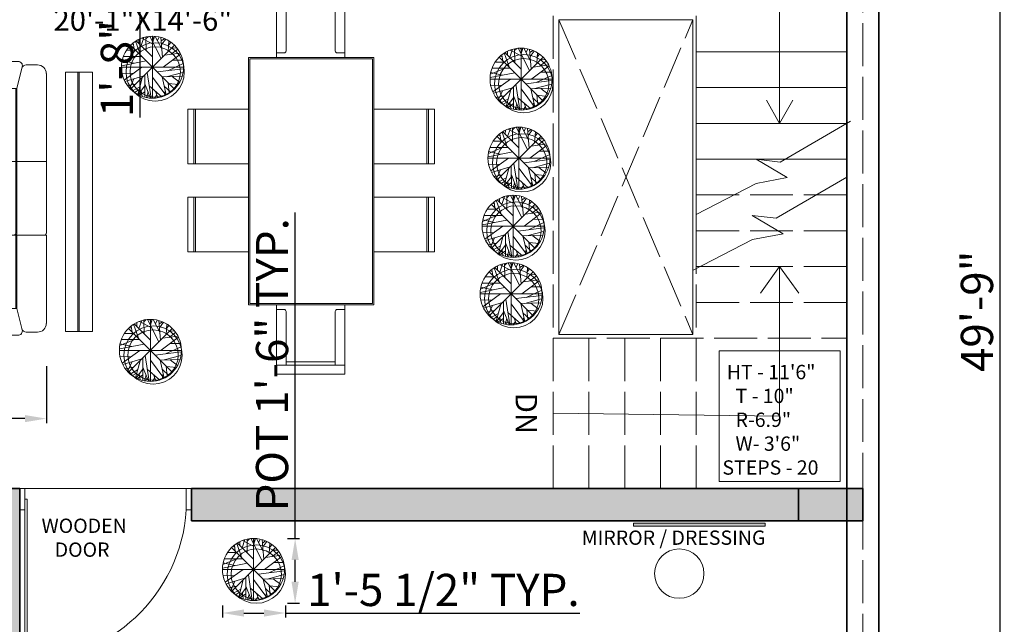
# Model space of a CAD drawing. Units: millimetres. Extents: x 595116 to 630915, y 909473 to 920225.
# Tile 132 of 134: x 630585 to 630860, y 919572 to 919741. Entities that reach past the tile are written whole.
import ezdxf

# ---------------------------------------------------------------- set-up
doc = ezdxf.new("R2010")
doc.units = ezdxf.units.MM
doc.linetypes.add('ACAD_ISO02W100', pattern=[15, 12, -3])
for name, color, linetype, lineweight in [('A-ANNO-SYMB', 7, 'Continuous', 18), ('A-AREA-IDEN', 7, 'Continuous', 20), ('A-FLOR-SCRN', 31, 'Continuous', 18), ('A-FLOR-STRS-HIDN', 142, 'ACAD_ISO02W100', 13), ('A-FURN', 32, 'Continuous', 18), ('A-WALL', 1, 'Continuous', 35), ('A-WALL-PATT', 8, 'Continuous', 13), ('C-PROP-REF', 240, 'ACAD_ISO02W100', 13), ('Column', 6, 'Continuous', 35), ('Dimension', 3, 'Continuous', 18), ('Doors', 31, 'Continuous', 20), ('L-PLNT', 85, 'Continuous', 13), ('STAIR CASE', 142, 'Continuous', 20), ('Text', 7, 'Continuous', 18)]:
    doc.layers.add(name, color=color, linetype=linetype, lineweight=lineweight)
doc.styles.get("Standard").update_dxf_attribs({"font": 'arial.ttf'})
doc.dimstyles.new('ISO-25', dxfattribs={"dimtxt": 9, "dimasz": 6, "dimexe": 1.25, "dimexo": 0.625, "dimtad": 1, "dimlunit": 4, "dimtxsty": 'Standard', "dimcen": 2.5, "dimadec": 0, "dimazin": 0, "dimtfac": 1, "dimtmove": 0, "dimatfit": 3, "dimfxl": 1, "dimarcsym": 0})

# ---------------------------------------------------------------- blocks, each defined once
blk = doc.blocks.new('KWD')
for points in [[(629753.63, 919957.93), (629752.54, 919957.93), (629752.54, 919953.43), (629753.63, 919953.43)], [(629787.45, 919957.93), (629787.45, 919953.43), (629788.54, 919953.43), (629788.54, 919957.93)]]:
    blk.add_lwpolyline(points, close=True)
blk.add_lwpolyline([(629753.63, 919921.79), (629753.63, 919955.68), (629754.13, 919955.68), (629754.13, 919921.8)])
blk.add_arc((629753.64, 919955.68), 33.88, 269.99, 356.196)
blk = doc.blocks.new('SOFA')
for p, q in [((629520.59, 919742.63), (629517.45, 919742.63)), ((629517.45, 919742.63), (629520.59, 919742.63)), ((629543.7, 919743.59), (629522.89, 919743.59)), ((629522.89, 919743.59), (629543.7, 919743.59)), ((629514.98, 919740.17), (629514.98, 919695.65)), ((629514.98, 919695.65), (629514.98, 919740.17)), ((629521.79, 919741.7), (629521.7, 919742.06)), ((629521.7, 919742.06), (629523.2, 919736.06)), ((629546.16, 919741.12), (629546.16, 919739.22)), ((629546.16, 919741.12), (629546.16, 919737.29)), ((629588.11, 919740.62), (629608.91, 919740.62)), ((629588.11, 919740.62), (629608.91, 919740.62)), ((629611.21, 919739.66), (629614.36, 919739.66)), ((629611.21, 919739.66), (629614.36, 919739.66)), ((629547.17, 919738.01), (629547.17, 919695.65)), ((629547.17, 919738.01), (629547.17, 919695.65)), ((629585.64, 919738.15), (629585.64, 919734.33)), ((629585.64, 919736.25), (629585.64, 919738.15)), ((629610.11, 919739.09), (629608.61, 919733.09)), ((629610.11, 919739.09), (629610.02, 919738.73)), ((629616.82, 919737.2), (629616.82, 919710.3)), ((629616.82, 919737.2), (629616.82, 919710.3)), ((629523.2, 919736.06), (629523.2, 919695.65)), ((629523.2, 919695.65), (629523.2, 919736.06)), ((629523.2, 919695.65), (629523.2, 919736.06)), ((629544.93, 919736.06), (629523.2, 919736.06)), ((629523.2, 919736.06), (629523.53, 919736.06)), ((629523.2, 919736.06), (629523.53, 919736.06)), ((629523.53, 919736.06), (629523.53, 919695.65)), ((629523.53, 919736.06), (629523.53, 919695.65)), ((629523.53, 919736.06), (629523.53, 919695.65)), ((629584.64, 919735.04), (629584.64, 919712.53)), ((629584.64, 919712.53), (629584.64, 919735.04)), ((629586.87, 919733.09), (629608.61, 919733.09)), ((629608.28, 919733.09), (629608.61, 919733.09)), ((629608.28, 919714.4), (629608.28, 919733.09)), ((629608.28, 919733.09), (629608.28, 919714.4)), ((629608.61, 919733.09), (629608.61, 919714.4)), ((629608.61, 919733.09), (629608.61, 919714.4)), ((629556.25, 919728.06), (629556.25, 919687.01)), ((629556.25, 919687.01), (629556.25, 919728.06)), ((629576.77, 919728.06), (629556.25, 919728.06)), ((629556.25, 919728.06), (629576.77, 919728.06)), ((629559.82, 919728), (629559.82, 919727.13)), ((629561.06, 919728), (629561.06, 919725.63)), ((629562.29, 919728), (629562.29, 919724.5)), ((629563.52, 919728), (629563.52, 919723.63)), ((629564.75, 919728), (629564.75, 919722.96)), ((629565.98, 919728), (629565.98, 919722.42)), ((629567.19, 919727.97), (629567.19, 919721.68)), ((629568.42, 919727.08), (629568.42, 919720.54)), ((629569.65, 919725.8), (629569.65, 919718.67)), ((629569.65, 919725.8), (629569.65, 919718.67)), ((629576.77, 919687.01), (629576.77, 919728.06)), ((629576.77, 919728.06), (629576.77, 919687.01)), ((629570.88, 919723.75), (629570.88, 919716.49)), ((629570.88, 919716.49), (629570.88, 919723.75)), ((629572.12, 919720.99), (629572.12, 919714.94)), ((629573.35, 919718.86), (629573.35, 919713.74)), ((629547.17, 919715.59), (629514.98, 919715.59)), ((629574.58, 919717.12), (629574.58, 919712.78)), ((629575.81, 919715.64), (629575.81, 919712.02)), ((629557.33, 919712.4), (629557.33, 919707.56)), ((629557.33, 919707.56), (629557.33, 919712.4)), ((629585.64, 919709.42), (629585.64, 919713.17)), ((629586.87, 919714.4), (629608.61, 919714.4)), ((629608.61, 919714.4), (629608.28, 919714.4)), ((629610.09, 919708.48), (629608.61, 919714.4)), ((629558.57, 919711.23), (629558.57, 919706.97)), ((629559.8, 919710.18), (629559.8, 919706.31)), ((629585.64, 919709.42), (629585.64, 919711.32)), ((629561.03, 919709.25), (629561.03, 919705.57)), ((629562.26, 919708.41), (629562.26, 919704.73)), ((629563.49, 919707.66), (629563.49, 919703.8)), ((629564.72, 919706.99), (629564.72, 919702.74)), ((629588.11, 919706.95), (629608.89, 919706.95)), ((629608.89, 919706.95), (629588.11, 919706.95)), ((629610.02, 919708.77), (629610.09, 919708.48)), ((629611.21, 919707.83), (629611.48, 919707.83)), ((629611.48, 919707.83), (629611.21, 919707.83)), ((629611.48, 919707.83), (629614.36, 919707.83)), ((629614.36, 919707.83), (629611.48, 919707.83)), ((629565.96, 919706.31), (629565.96, 919701.75)), ((629567.19, 919705.56), (629567.19, 919701.12)), ((629568.42, 919704.73), (629568.42, 919700.78)), ((629569.65, 919703.81), (629569.65, 919700.45)), ((629570.88, 919702.8), (629570.88, 919699.98)), ((629572.12, 919701.68), (629572.12, 919699.37)), ((629573.35, 919700.43), (629573.35, 919698.59)), ((629574.58, 919699.04), (629574.58, 919697.6)), ((629575.81, 919697.48), (629575.81, 919696.34)), ((629575.81, 919697.48), (629575.81, 919696.34)), ((629547.17, 919695.06), (629514.98, 919695.06)), ((629514.98, 919695.06), (629514.98, 919670.42)), ((629514.98, 919670.42), (629514.98, 919695.06)), ((629514.98, 919695.06), (629515.44, 919695.06)), ((629515.6, 919695.04), (629546.55, 919695.04)), ((629523.2, 919695.06), (629523.2, 919674.53)), ((629523.2, 919674.53), (629523.2, 919695.04)), ((629523.2, 919674.53), (629523.2, 919695.04)), ((629523.2, 919695.04), (629523.53, 919695.04)), ((629523.2, 919695.04), (629523.53, 919695.04)), ((629523.53, 919695.04), (629523.53, 919695.11)), ((629523.53, 919695.04), (629523.53, 919695.11)), ((629523.53, 919695.06), (629523.53, 919674.53)), ((629523.53, 919695.04), (629523.53, 919674.53)), ((629523.53, 919695.04), (629523.53, 919674.53)), ((629524.14, 919695.04), (629523.53, 919695.04)), ((629524.14, 919695.04), (629523.53, 919695.04)), ((629546.71, 919695.06), (629547.17, 919695.06)), ((629547.17, 919695.06), (629547.17, 919672.66)), ((629547.17, 919695.06), (629547.17, 919672.66)), ((629585.64, 919690.3), (629585.64, 919688.39)), ((629585.64, 919690.3), (629585.64, 919686.55)), ((629588.11, 919692.76), (629608.89, 919692.76)), ((629608.89, 919692.76), (629588.11, 919692.76)), ((629610.09, 919691.23), (629608.61, 919685.31)), ((629610.02, 919690.95), (629610.09, 919691.23)), ((629611.21, 919691.88), (629611.48, 919691.88)), ((629611.48, 919691.88), (629611.21, 919691.88)), ((629611.48, 919691.88), (629614.36, 919691.88)), ((629614.36, 919691.88), (629611.48, 919691.88)), ((629616.82, 919662.52), (629616.82, 919689.42)), ((629616.82, 919662.52), (629616.82, 919689.42)), ((629556.25, 919687.01), (629576.77, 919687.01)), ((629576.77, 919687.01), (629556.25, 919687.01)), ((629584.64, 919664.68), (629584.64, 919687.18)), ((629584.64, 919687.18), (629584.64, 919664.68)), ((629586.87, 919685.31), (629608.61, 919685.31)), ((629608.61, 919685.31), (629608.28, 919685.31)), ((629608.28, 919685.31), (629608.28, 919666.62)), ((629608.28, 919666.62), (629608.28, 919685.31)), ((629608.61, 919666.62), (629608.61, 919685.31)), ((629608.61, 919666.62), (629608.61, 919685.31)), ((629521.72, 919668.61), (629523.2, 919674.53)), ((629544.93, 919674.53), (629523.2, 919674.53)), ((629523.53, 919674.53), (629523.2, 919674.53)), ((629523.53, 919674.53), (629523.2, 919674.53)), ((629546.16, 919669.54), (629546.16, 919673.3)), ((629546.16, 919671.45), (629546.16, 919669.54)), ((629521.72, 919668.61), (629521.79, 919668.89)), ((629520.32, 919667.96), (629517.45, 919667.96)), ((629520.32, 919667.96), (629517.45, 919667.96)), ((629520.59, 919667.96), (629520.32, 919667.96)), ((629520.59, 919667.96), (629520.32, 919667.96)), ((629543.7, 919667.08), (629522.91, 919667.08)), ((629543.7, 919667.08), (629522.91, 919667.08)), ((629585.64, 919661.56), (629585.64, 919665.39)), ((629586.87, 919666.62), (629608.61, 919666.62)), ((629608.28, 919666.62), (629608.61, 919666.62)), ((629610.11, 919660.63), (629608.61, 919666.62)), ((629585.64, 919663.47), (629585.64, 919661.56)), ((629610.11, 919660.63), (629610.02, 919660.99)), ((629611.21, 919660.05), (629614.36, 919660.05)), ((629611.21, 919660.05), (629614.36, 919660.05)), ((629588.11, 919659.1), (629608.91, 919659.1)), ((629588.11, 919659.1), (629608.91, 919659.1))]:
    blk.add_line(p, q)
for centre, radius, start, end in [((629517.45, 919740.17), 2.46, 90, 180), ((629517.45, 919740.17), 2.46, 90, 180), ((629520.59, 919741.4), 1.23, 14.0362, 90), ((629520.59, 919741.4), 1.23, 14.0362, 90), ((629522.89, 919742.36), 1.23, 90, 194.0362), ((629522.89, 919742.36), 1.23, 90, 194.0362), ((629543.7, 919741.12), 2.46, 0, 90), ((629543.7, 919741.12), 2.46, 0, 90), ((629588.11, 919738.15), 2.46, 90, 180), ((629588.11, 919738.15), 2.46, 90, 180), ((629608.91, 919739.39), 1.23, 345.9638, 90), ((629608.91, 919739.39), 1.23, 345.9638, 90), ((629611.21, 919738.43), 1.23, 90, 165.9638), ((629611.21, 919738.43), 1.23, 90, 165.9638), ((629614.36, 919737.2), 2.46, 0, 90), ((629614.36, 919737.2), 2.46, 0, 90), ((629544.93, 919737.29), 1.23, 270, 0), ((629545.94, 919738.01), 1.23, 0, 90), ((629545.94, 919738.01), 1.23, 0, 79.4007), ((629585.87, 919735.04), 1.23, 90, 180), ((629585.87, 919735.04), 1.23, 100.5993, 180), ((629586.87, 919734.33), 1.23, 180, 270), ((629570.11, 919734.3), 12.54, 210.2644, 248.0021), ((629562.37, 919720.03), 9.29, 21.2599, 58.8091), ((629562.37, 919720.03), 9.29, 23.6102, 38.4008), ((629594.57, 919732.56), 25.26, 201.2599, 225.1217), ((629562.42, 919715.26), 7.99, 24.8088, 68.0021), ((629582.84, 919724.7), 14.51, 204.5645, 214.4539), ((629582.84, 919724.7), 14.51, 204.8088, 245.1378), ((629577.93, 919732.79), 28.98, 222.2366, 242.5747), ((629577.93, 919732.79), 28.98, 224.7026, 242.5747), ((629585.87, 919712.53), 1.23, 180, 270), ((629585.87, 919712.53), 1.23, 180, 259.4007), ((629586.87, 919713.17), 1.23, 90, 180), ((629588.11, 919709.42), 2.46, 180, 270), ((629588.11, 919709.42), 2.46, 180, 270), ((629614.36, 919710.3), 2.46, 270, 0), ((629614.36, 919710.3), 2.46, 270, 0), ((629546.11, 919682.25), 27.68, 46.9747, 68.4773), ((629546.11, 919682.25), 27.68, 46.9747, 66.0851), ((629549.56, 919678.1), 32.63, 33.5604, 62.5747), ((629549.56, 919678.1), 32.63, 36.4252, 62.5747), ((629608.89, 919708.18), 1.23, 270, 14.0362), ((629608.89, 919708.18), 1.23, 270, 14.0362), ((629611.21, 919709.06), 1.23, 194.0362, 270), ((629611.21, 919709.06), 1.23, 194.0362, 270), ((629569.57, 919707.39), 6.7, 226.9747, 258.3827), ((629569.57, 919707.39), 6.7, 226.9746, 258.3828), ((629565.49, 919687.55), 13.55, 33.8658, 78.3827), ((629565.49, 919687.55), 13.55, 40.4201, 78.3827), ((629515.6, 919695.65), 0.616, 180, 270), ((629515.6, 919695.65), 0.616, 180, 255.079), ((629523.81, 919695.65), 0.616, 180, 270), ((629523.81, 919695.65), 0.616, 180, 242.2854), ((629523.81, 919695.65), 0.616, 180, 242.2854), ((629524.14, 919695.65), 0.616, 180, 270), ((629524.14, 919695.65), 0.616, 180, 270), ((629524.14, 919695.65), 0.616, 180, 270), ((629546.55, 919695.65), 0.616, 270, 0), ((629546.55, 919695.65), 0.616, 284.921, 0), ((629588.11, 919690.3), 2.46, 90, 180), ((629588.11, 919690.3), 2.46, 90, 180), ((629608.89, 919691.53), 1.23, 345.9638, 90), ((629608.89, 919691.53), 1.23, 345.9638, 90), ((629611.21, 919690.65), 1.23, 90, 165.9638), ((629611.21, 919690.65), 1.23, 90, 165.9638), ((629614.36, 919689.42), 2.46, 0, 90), ((629614.36, 919689.42), 2.46, 0, 90), ((629585.87, 919687.18), 1.23, 90, 180), ((629585.87, 919687.18), 1.23, 100.5993, 180), ((629586.87, 919686.55), 1.23, 180, 270), ((629544.93, 919673.3), 1.23, 0, 90), ((629545.94, 919672.66), 1.23, 270, 0), ((629545.94, 919672.66), 1.23, 280.5993, 0), ((629517.45, 919670.42), 2.46, 180, 270), ((629517.45, 919670.42), 2.46, 180, 270), ((629520.59, 919669.19), 1.23, 270, 345.9638), ((629520.59, 919669.19), 1.23, 270, 345.9638), ((629522.91, 919668.31), 1.23, 165.9638, 270), ((629522.91, 919668.31), 1.23, 165.9638, 270), ((629543.7, 919669.54), 2.46, 270, 0), ((629543.7, 919669.54), 2.46, 270, 0), ((629586.87, 919665.39), 1.23, 90, 180), ((629585.87, 919664.68), 1.23, 180, 270), ((629585.87, 919664.68), 1.23, 180, 259.4007), ((629588.11, 919661.56), 2.46, 180, 270), ((629588.11, 919661.56), 2.46, 180, 270), ((629608.91, 919660.33), 1.23, 270, 14.0362), ((629608.91, 919660.33), 1.23, 270, 14.0362), ((629611.21, 919661.28), 1.23, 194.0362, 270), ((629611.21, 919661.28), 1.23, 194.0362, 270), ((629614.36, 919662.52), 2.46, 270, 0), ((629614.36, 919662.52), 2.46, 270, 0)]:
    blk.add_arc(centre, radius, start, end)
at = {"flags": 9}
for tag in ['XSIZE', 'YSIZE']:
    blk.add_attdef(tag, (629556.25, 919728.06), '', height=0.0205, rotation=270, dxfattribs=at)
blk = doc.blocks.new('DINING')
for p, q in [((630176.61, 919568.69), (630176.61, 919601.05)), ((630176.61, 919601.05), (630208.41, 919601.05)), ((630208.41, 919601.05), (630208.41, 919568.69)), ((630176.61, 919596.78), (630208.41, 919596.78)), ((630181.05, 919571.76), (630181.05, 919596.78)), ((630203.97, 919571.76), (630203.97, 919596.78)), ((630181.05, 919595.21), (630203.97, 919595.21)), ((630163.47, 919568.69), (630222.04, 919568.69)), ((630163.47, 919453.21), (630163.47, 919568.69)), ((630164.11, 919568.05), (630221.39, 919568.05)), ((630164.11, 919453.85), (630164.11, 919568.05)), ((630176.61, 919570.82), (630180.11, 919570.82)), ((630208.41, 919570.82), (630204.91, 919570.82)), ((630221.39, 919568.05), (630221.39, 919453.85)), ((630222.04, 919568.69), (630222.04, 919453.21)), ((630163.47, 919544.57), (630135.12, 919544.57)), ((630135.12, 919544.57), (630135.12, 919519)), ((630137.93, 919544.57), (630137.93, 919519)), ((630138.72, 919544.57), (630138.72, 919519)), ((630222.04, 919544.57), (630250.39, 919544.57)), ((630246.79, 919544.57), (630246.79, 919519)), ((630247.58, 919544.57), (630247.58, 919519)), ((630250.39, 919544.57), (630250.39, 919519)), ((630135.12, 919519), (630163.47, 919519)), ((630250.39, 919519), (630222.04, 919519)), ((630163.47, 919503.52), (630135.12, 919503.52)), ((630135.12, 919503.52), (630135.12, 919477.96)), ((630137.93, 919503.52), (630137.93, 919477.96)), ((630138.72, 919503.52), (630138.72, 919477.96)), ((630222.04, 919503.52), (630250.39, 919503.52)), ((630246.79, 919503.52), (630246.79, 919477.96)), ((630247.58, 919503.52), (630247.58, 919477.96)), ((630250.39, 919503.52), (630250.39, 919477.96)), ((630135.12, 919477.96), (630163.47, 919477.96)), ((630250.39, 919477.96), (630222.04, 919477.96)), ((630222.04, 919453.21), (630163.47, 919453.21)), ((630221.39, 919453.85), (630164.11, 919453.85)), ((630176.61, 919453.21), (630176.61, 919420.86)), ((630208.41, 919420.86), (630208.41, 919453.21)), ((630176.61, 919451.09), (630180.11, 919451.09)), ((630181.05, 919450.14), (630181.05, 919425.13)), ((630203.97, 919450.14), (630203.97, 919425.13)), ((630208.41, 919451.09), (630204.91, 919451.09)), ((630181.05, 919426.7), (630203.97, 919426.7)), ((630176.61, 919425.13), (630208.41, 919425.13)), ((630176.61, 919420.86), (630208.41, 919420.86))]:
    blk.add_line(p, q)
for centre, start, end in [((630180.11, 919571.76), 270, 0), ((630204.91, 919571.76), 180, 270), ((630180.11, 919450.14), 0, 90), ((630204.91, 919450.14), 90, 180)]:
    blk.add_arc(centre, 0.945, start, end)
blk = doc.blocks.new('*D131')
at = {"layer": 'Defpoints', "color": 0, "transparency": 16777216}
for p in [(630820.1, 919957.93), (630820.1, 919360.93), (630858.37, 919360.93)]:
    blk.add_point(p, dxfattribs=at)
at = {"layer": 'Dimension', "color": 0, "lineweight": -2, "transparency": 16777216}
for p, q in [((630820.72, 919957.93), (630859.62, 919957.93)), ((630858.37, 919951.93), (630858.37, 919366.93)), ((630820.72, 919360.93), (630859.62, 919360.93))]:
    blk.add_line(p, q, dxfattribs=at)
at = {"layer": 'Dimension', "color": 0, "transparency": 16777216}
for points in [[(630857.37, 919951.93), (630859.37, 919951.93), (630858.37, 919957.93)], [(630857.37, 919366.93), (630859.37, 919366.93), (630858.37, 919360.93)]]:
    blk.add_solid(points, dxfattribs=at)
at = {"layer": 'Dimension', "color": 0, "transparency": 16777216, "insert": (630853.15, 919659.43), "char_height": 9, "attachment_point": 5, "rotation": 90}
blk.add_mtext('49\'-9"', dxfattribs=at)
blk = doc.blocks.new('POTTED-PLANT')
for p, q in [((3.96, 16.73), (5.31, 12.84)), ((4.16, 16.82), (8.64, 12.35)), ((4.85, 16.17), (4.88, 17.22)), ((5.49, 15.52), (6.28, 17.77)), ((5.61, 17.51), (8.67, 15.94)), ((6.86, 17.38), (7.52, 18.03)), ((6.89, 14.08), (6.86, 17.93)), ((7.9, 18.06), (11.06, 11.86)), ((9.02, 17.38), (8.46, 18.1)), ((8.67, 18.11), (8.67, 0.76)), ((8.74, 16.47), (9.2, 18.06)), ((11.32, 14.57), (9.46, 18.06)), ((10.09, 16.89), (10.53, 17.9)), ((11.52, 12.26), (11.04, 17.77)), ((11.14, 16.82), (12.03, 17.41)), ((11.24, 15.75), (12.36, 17.28)), ((13.25, 16.79), (13.05, 13.86)), ((1.47, 14.18), (3.93, 14.18)), ((14.75, 15.51), (2.6, 3.36)), ((14.75, 3.36), (2.6, 15.51)), ((2.87, 15.88), (3.4, 15.68)), ((3.32, 16.24), (3.58, 14.57)), ((13.17, 15.58), (13.86, 16.4)), ((13.91, 13.07), (15.74, 14.51)), ((14.04, 14.8), (15.41, 14.87)), ((0.04, 9.84), (6.94, 11.18)), ((4.01, 12.42), (0.12, 10.79)), ((0.19, 11.28), (3.48, 10.53)), ((0.57, 12.45), (5.66, 12.45)), ((16.53, 13.1), (11.7, 9.48)), ((12.05, 12.81), (16.38, 13.4)), ((14.24, 11.38), (17.09, 11.41)), ((0, 9.44), (17.35, 9.44)), ((0.78, 5.86), (5.74, 9.45)), ((10.02, 8.11), (17.3, 9.03)), ((12.92, 8.47), (17.27, 10.46)), ((0.22, 7.66), (3.4, 7.75)), ((0.98, 5.47), (6.25, 7.04)), ((3.48, 6.19), (2.31, 3.58)), ((5.79, 6.51), (4.54, 1.82)), ((6.53, 7.26), (6.56, 1.1)), ((7.22, 7.98), (8.31, 0.8)), ((8.67, 6.68), (12.41, 1.65)), ((11.37, 6.74), (12.54, 1.72)), ((11.39, 6.74), (16.97, 6.94)), ((12.49, 6.77), (17.19, 8.01)), ((14.19, 6.81), (16.25, 5.24)), ((3.99, 4.75), (1.72, 4.29)), ((5.1, 3.97), (3.07, 2.83)), ((4.88, 3.09), (3.65, 2.4)), ((6.56, 4.2), (4.67, 1.78)), ((5.56, 2.86), (5.79, 1.33)), ((6.56, 4.78), (8.11, 0.84)), ((7.78, 4.2), (11.26, 1.2)), ((11.98, 4.16), (13.78, 2.43)), ((12.26, 2.96), (12, 1.49)), ((13.07, 5.08), (13.35, 2.21)), ((13.22, 4.91), (15.85, 4.62)), ((6.56, 2.6), (5.05, 1.59)), ((7.45, 2.57), (7.01, 0.97)), ((7.75, 1.82), (7.32, 0.93)), ((9.89, 1.75), (9.23, 0.84)), ((9.53, 2.7), (10.2, 0.97))]:
    blk.add_line(p, q)
for centre, radius in [((8.67, 9.44), 8.67), ((9.43, 8.14), 8.14), ((9.43, 8.14), 7.03)]:
    blk.add_circle(centre, radius)
blk = doc.blocks.new('COLUMN-RECT-18X9')
h = blk.add_hatch(color=256)
h.dxf.hatch_style = 1
h.paths.add_polyline_path([(18, 9), (0, 9), (0, 0), (18, 0)])
blk.add_lwpolyline([(0, 9), (18, 9), (18, 0), (0, 0)], close=True)
blk = doc.blocks.new('*D171')
at = {"layer": 'Defpoints', "color": 0, "transparency": 16777216}
for p in [(630621.34, 919794.96), (630618.13, 919774.78), (630621.34, 919774.78)]:
    blk.add_point(p, dxfattribs=at)
at = {"layer": 'Dimension', "color": 0, "lineweight": -2, "transparency": 16777216}
for p, q in [((630620.72, 919794.96), (630616.88, 919794.96)), ((630618.13, 919788.96), (630618.13, 919780.78)), ((630620.72, 919774.78), (630616.88, 919774.78)), ((630618.13, 919774.78), (630618.13, 919713.52))]:
    blk.add_line(p, q, dxfattribs=at)
at = {"layer": 'Dimension', "color": 0, "transparency": 16777216}
for points in [[(630617.13, 919788.96), (630619.13, 919788.96), (630618.13, 919794.96)], [(630617.13, 919780.78), (630619.13, 919780.78), (630618.13, 919774.78)]]:
    blk.add_solid(points, dxfattribs=at)
at = {"layer": 'Dimension', "color": 0, "transparency": 16777216, "insert": (630612.91, 919741.15), "char_height": 9, "attachment_point": 5, "rotation": 90}
blk.add_mtext('1\'-8" TYP.', dxfattribs=at)
blk = doc.blocks.new('*D182')
at = {"layer": 'Defpoints', "color": 0, "transparency": 16777216}
for p in [(630490.2, 919644.73), (630592.04, 919644.73), (630490.2, 919629.46)]:
    blk.add_point(p, dxfattribs=at)
at = {"layer": 'Dimension', "color": 0, "lineweight": -2, "transparency": 16777216}
for p, q in [((630490.2, 919644.11), (630490.2, 919628.21)), ((630592.04, 919644.11), (630592.04, 919628.21)), ((630490.2, 919629.46), (630340.81, 919629.46)), ((630586.04, 919629.46), (630496.2, 919629.46))]:
    blk.add_line(p, q, dxfattribs=at)
at = {"layer": 'Dimension', "color": 0, "transparency": 16777216}
for points in [[(630496.2, 919630.46), (630496.2, 919628.46), (630490.2, 919629.46)], [(630586.04, 919630.46), (630586.04, 919628.46), (630592.04, 919629.46)]]:
    blk.add_solid(points, dxfattribs=at)
at = {"layer": 'Dimension', "color": 0, "transparency": 16777216, "insert": (630412.5, 919634.74), "char_height": 9, "attachment_point": 5}
blk.add_mtext('SOFA GROUP 8\'-6" TYP.', dxfattribs=at)
blk = doc.blocks.new('*D206')
at = {"layer": 'Defpoints', "color": 0, "transparency": 16777216}
for p in [(630658.82, 919595.98), (630661.53, 919595.98), (630658.82, 919577.87)]:
    blk.add_point(p, dxfattribs=at)
at = {"layer": 'Dimension', "color": 0, "lineweight": -2, "transparency": 16777216}
for p, q in [((630661.53, 919595.98), (630661.53, 919686.98)), ((630659.44, 919595.98), (630662.78, 919595.98)), ((630661.53, 919583.87), (630661.53, 919589.98)), ((630659.44, 919577.87), (630662.78, 919577.87))]:
    blk.add_line(p, q, dxfattribs=at)
at = {"layer": 'Dimension', "color": 0, "transparency": 16777216}
for points in [[(630660.53, 919589.98), (630662.53, 919589.98), (630661.53, 919595.98)], [(630660.53, 919583.87), (630662.53, 919583.87), (630661.53, 919577.87)]]:
    blk.add_solid(points, dxfattribs=at)
at = {"layer": 'Dimension', "color": 0, "transparency": 16777216, "insert": (630656.25, 919644.48), "char_height": 9, "attachment_point": 5, "rotation": 90}
blk.add_mtext('POT 1\'-6" TYP.', dxfattribs=at)
blk = doc.blocks.new('*D207')
at = {"layer": 'Defpoints', "color": 0, "transparency": 16777216}
for p in [(630641.24, 919577.87), (630658.82, 919577.87), (630658.82, 919575.15)]:
    blk.add_point(p, dxfattribs=at)
at = {"layer": 'Dimension', "color": 0, "lineweight": -2, "transparency": 16777216}
for p, q in [((630641.24, 919577.25), (630641.24, 919573.9)), ((630647.24, 919575.15), (630652.82, 919575.15)), ((630658.82, 919577.25), (630658.82, 919573.9)), ((630658.82, 919575.15), (630741.05, 919575.15))]:
    blk.add_line(p, q, dxfattribs=at)
at = {"layer": 'Dimension', "color": 0, "transparency": 16777216}
for points in [[(630647.24, 919576.15), (630647.24, 919574.15), (630641.24, 919575.15)], [(630652.82, 919576.15), (630652.82, 919574.15), (630658.82, 919575.15)]]:
    blk.add_solid(points, dxfattribs=at)
at = {"layer": 'Dimension', "color": 0, "transparency": 16777216, "insert": (630702.94, 919580.43), "char_height": 9, "attachment_point": 5}
blk.add_mtext('1\'-5 1/2" TYP.', dxfattribs=at)

msp = doc.modelspace()

# ---------------------------------------------------------------- hatches: boundary and pattern name
at = {"layer": 'A-FLOR-SCRN'}
h = msp.add_hatch(color=256, dxfattribs=at)
h.dxf.hatch_style = 1
h.paths.add_polyline_path([(630600.846, 919726.206), (630601.176, 919726.206), (630601.176, 919653.755), (630600.846, 919653.755)])
at = {"layer": 'A-FURN'}
h = msp.add_hatch(color=256, dxfattribs=at)
h.dxf.hatch_style = 1
h.paths.add_polyline_path([(630792.868, 919600.264), (630756.021, 919600.264), (630756.021, 919599.365), (630792.868, 919599.365)])
at = {"layer": 'A-WALL-PATT'}
h = msp.add_hatch(color=256, dxfattribs=at)
h.dxf.hatch_style = 1
h.paths.add_polyline_path([(630584.596, 919609.928), (630577.096, 919609.928), (630577.096, 919591.928), (630575.596, 919591.928), (630575.596, 919552.928), (630533.596, 919552.928), (630533.596, 919548.428), (630575.596, 919548.428), (630575.596, 919429.928), (630577.096, 919429.928), (630577.096, 919411.928), (630608.596, 919411.928), (630608.596, 919420.928), (630584.596, 919420.928)])
h = msp.add_hatch(color=256, dxfattribs=at)
h.dxf.hatch_style = 1
h.paths.add_polyline_path([(630802.096, 919609.928), (630632.596, 919609.928), (630632.596, 919603.928), (630632.596, 919600.928), (630802.096, 919600.928)])

# ---------------------------------------------------------------- linework, layer by layer
at = {"layer": 'A-ANNO-SYMB'}
for p, q in [((630796.86, 919762.246), (630796.86, 919711.928)), ((630796.86, 919711.928), (630793.192, 919718.393)), ((630796.86, 919711.928), (630800.527, 919718.393)), ((630796.86, 919671.928), (630791.492, 919664.483)), ((630796.86, 919630.106), (630796.86, 919671.928)), ((630796.86, 919671.928), (630802.227, 919664.483)), ((630733.596, 919630.928), (630796.86, 919630.106))]:
    msp.add_line(p, q, dxfattribs=at)
msp.add_lwpolyline([(630779.986, 919648.35), (630813.733, 919648.35), (630813.733, 919611.862), (630779.986, 919611.862)], close=True, dxfattribs=at)
at = {"layer": 'A-FLOR-SCRN'}
for p, q in [((630600.846, 919726.206), (630600.846, 919653.755)), ((630601.176, 919726.206), (630601.176, 919653.755))]:
    msp.add_line(p, q, dxfattribs=at)
msp.add_lwpolyline([(630604.92, 919726.206), (630597.432, 919726.206), (630597.432, 919653.755), (630604.92, 919653.755)], close=True, dxfattribs=at)
at = {"layer": 'A-FLOR-STRS-HIDN'}
for p, q in [((630733.596, 919741.928), (630733.596, 919651.928)), ((630735.225, 919740.877), (630772.632, 919652.945)), ((630735.225, 919652.945), (630772.632, 919740.877)), ((630773.596, 919691.928), (630815.596, 919691.928)), ((630773.596, 919681.928), (630815.596, 919681.928)), ((630773.596, 919681.928), (630773.596, 919609.928)), ((630773.596, 919671.928), (630815.596, 919671.928)), ((630773.596, 919661.928), (630815.596, 919661.928)), ((630733.596, 919651.928), (630815.596, 919651.928)), ((630733.596, 919651.928), (630733.596, 919609.928)), ((630743.596, 919651.928), (630743.596, 919609.928)), ((630753.596, 919651.928), (630753.596, 919609.928)), ((630763.596, 919651.928), (630763.596, 919609.928))]:
    msp.add_line(p, q, dxfattribs=at)
at = {"layer": 'A-FURN'}
msp.add_lwpolyline([(630756.021, 919600.264), (630792.868, 919600.264), (630792.868, 919599.365), (630756.021, 919599.365)], close=True, dxfattribs=at)
msp.add_circle((630768.828, 919586.157), 6.897, dxfattribs=at)
at = {"layer": 'A-WALL'}
for p, q in [((630815.596, 920020.393), (630815.596, 919333.928)), ((630575.596, 919609.928), (630584.596, 919609.928)), ((630584.596, 919420.928), (630584.596, 919609.928)), ((630632.596, 919600.928), (630632.596, 919609.928)), ((630632.596, 919609.928), (630820.096, 919609.928)), ((630632.596, 919600.928), (630820.096, 919600.928))]:
    msp.add_line(p, q, dxfattribs=at)
msp.add_lwpolyline([(630824.596, 920020.393), (630824.596, 919333.928)], dxfattribs=at)
at = {"layer": 'C-PROP-REF'}
msp.add_line((630820.096, 920084.928), (630820.096, 919150.928), dxfattribs=at)
at = {"layer": 'Doors'}
msp.add_line((630586.054, 919609.928), (630631.139, 919609.928), dxfattribs=at)
at = {"layer": 'STAIR CASE'}
for p, q in [((630773.596, 919681.928), (630773.596, 919741.928)), ((630773.596, 919731.928), (630815.596, 919731.928)), ((630773.596, 919721.928), (630815.596, 919721.928)), ((630773.596, 919711.928), (630815.596, 919711.928)), ((630773.596, 919701.928), (630815.596, 919701.928))]:
    msp.add_line(p, q, dxfattribs=at)
msp.add_lwpolyline([(630735.225, 919740.877), (630772.632, 919740.877), (630772.632, 919652.945), (630735.225, 919652.945)], close=True, dxfattribs=at)
for points in [[(630773.596, 919686.489), (630790.32, 919695.169), (630798.947, 919696.774), (630790.294, 919701.928), (630797.014, 919701.125), (630816.672, 919712.564)], [(630772.52, 919670.779), (630789.244, 919679.46), (630797.871, 919681.064), (630789.218, 919686.218), (630795.938, 919685.416), (630815.596, 919696.855)]]:
    msp.add_lwpolyline(points, dxfattribs=at)

# ---------------------------------------------------------------- block references
at = {"layer": 'A-FURN', "xscale": 0.5984731567659999, "yscale": 0.5984731567659999, "zscale": 0.5984731567659999}
msp.add_blockref('DINING', (253512.563, 369393.149), dxfattribs=at)
at = {"layer": 'A-FURN', "xscale": -1}
msp.add_blockref('SOFA', (1260107.02, -14.364), dxfattribs=at)
at = {"layer": 'Column'}
msp.add_blockref('COLUMN-RECT-18X9', (630802.096, 919600.928), dxfattribs=at)
at = {"layer": 'Doors', "xscale": 1.333333333333333, "yscale": 1.333333333333333, "zscale": 1.333333333333333}
msp.add_blockref('KWD', (-209085.458, -307000.643), dxfattribs=at)
at = {"layer": 'L-PLNT'}
for p in [(630613.012, 919718.163), (630715.971, 919714.849), (630715.389, 919692.758), (630713.763, 919673.73), (630713.181, 919654.855), (630612.43, 919639.068), (630641.243, 919577.87)]:
    msp.add_blockref('POTTED-PLANT', p, dxfattribs=at)

# ---------------------------------------------------------------- texts
at = {"layer": 'A-ANNO-SYMB', "insert": (630777.213, 919644.466), "char_height": 4, "attachment_point": 1}
msp.add_mtext_dynamic_manual_height_columns('{    HT - 11\'6"\\P      T - 10"\\P      R-6.9"\\P      W- 3\'6"\\P   STEPS - 20}', width=61.33456, gutter_width=12.5, heights=[0], dxfattribs=at)
at = {"layer": 'A-ANNO-SYMB', "insert": (630729.112, 919645.837), "char_height": 6, "attachment_point": 1, "rotation": 270}
msp.add_mtext_dynamic_manual_height_columns('{     DN}', width=61.33456, gutter_width=12.5, heights=[0], dxfattribs=at)
at = {"layer": 'A-AREA-IDEN', "insert": (630590.357, 919753.787), "char_height": 6, "attachment_point": 1}
msp.add_mtext_dynamic_manual_height_columns('{      LOBBY\\P  20\'-1"X14\'-6"}', width=83.57324, gutter_width=12.5, heights=[0], dxfattribs=at)
at = {"layer": 'Text', "char_height": 4, "attachment_point": 1}
for s, width, insert in [('{     WOODEN\\P        DOOR}', 61.33456, (630584.596, 919601.518)), ('{     MIRROR / DRESSING}', 72.55106, (630735.485, 919598.196))]:
    msp.add_mtext_dynamic_manual_height_columns(s, width=width, gutter_width=12.5, heights=[0], dxfattribs=dict(at, insert=insert))

# ---------------------------------------------------------------- dimensions: what is measured, and where the dimension line sits
at = {"layer": 'Dimension'}
dim = msp.add_linear_dim(base=(630858.371, 919360.928), p1=(630820.096, 919957.928), p2=(630820.096, 919360.928), angle=90, dimstyle='ISO-25', override={"dimclrd": 0, "dimclre": 0, "dimclrt": 0}, dxfattribs=at)
dim.commit()
dim.dimension.update_dxf_attribs({"geometry": '*D131', "text_midpoint": (630853.151, 919659.428)})
for base, p1, p2, angle, text, picture, middle in [((630618.131, 919774.777), (630621.342, 919794.957), (630621.342, 919774.777), 270, '<> TYP.', '*D171', (630612.911, 919741.146)), ((630661.535, 919595.981), (630658.818, 919577.871), (630658.818, 919595.981), 90, 'POT <> TYP.', '*D206', (630656.253, 919644.481)), ((630490.198, 919629.458), (630592.035, 919644.733), (630490.198, 919644.733), 180, 'SOFA GROUP <> TYP.', '*D182', (630412.503, 919634.739))]:
    dim = msp.add_linear_dim(base=base, p1=p1, p2=p2, angle=angle, text=text, dimstyle='ISO-25', override={"dimdec": 1, "dimlfac": 1, "dimrnd": 0, "dimzin": 1, "dimdsep": 46, "dimlunit": 4, "dimfrac": 2}, dxfattribs=at)
    dim.commit()
    dim.dimension.update_dxf_attribs({"geometry": picture, "text_midpoint": middle})
dim = msp.add_linear_dim(base=(630658.818, 919575.154), p1=(630641.243, 919577.871), p2=(630658.818, 919577.871), text='<> TYP.', dimstyle='ISO-25', override={"dimdec": 1, "dimlfac": 1, "dimrnd": 0, "dimzin": 1, "dimdsep": 46, "dimlunit": 4, "dimfrac": 2}, dxfattribs=at)
dim.commit()
dim.dimension.update_dxf_attribs({"geometry": '*D207', "text_midpoint": (630702.935, 919580.433)})

doc.saveas('drawing.dxf')
